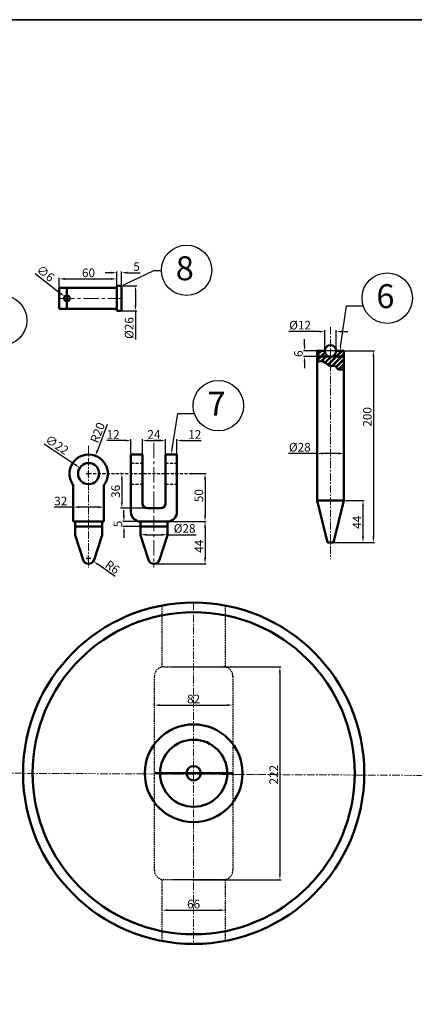
# Model space of a CAD drawing. Units: millimetres. Extents: x -282 to 2335, y -1129 to 664.
# Tile 7 of 8: x 1341 to 1752, y -363 to 664. Entities that reach past the tile are written whole.
import ezdxf
from ezdxf import colors
from ezdxf.entities.mleader import LeaderData, LeaderLine
from ezdxf.math import Vec2, Vec3

# ---------------------------------------------------------------- set-up
doc = ezdxf.new("R2010")
doc.units = ezdxf.units.MM
doc.header["$LTSCALE"] = 0.5
doc.linetypes.add('CENTER', pattern=[50.8, 31.75, -6.35, 6.35, -6.35])
doc.linetypes.add('HIDDEN', pattern=[9.525, 6.35, -3.175])
for name, color, linetype, lineweight in [('M-CNTR', 1, 'CENTER', 18), ('M-DIMS', 2, 'Continuous', 25), ('M-HATC', 8, 'Continuous', 18), ('M-HIDN', 4, 'HIDDEN', 25), ('M-OUTL', 7, 'Continuous', 50), ('M-TEXT', 3, 'Continuous', 25), ('M-TTLB', 7, 'Continuous', 35)]:
    doc.layers.add(name, color=color, linetype=linetype, lineweight=lineweight)
doc.styles.get("Standard").update_dxf_attribs({"font": 'arial.ttf'})
doc.dimstyles.new('ISO-25', dxfattribs={"dimtxt": 9, "dimasz": 6, "dimexe": 1.25, "dimexo": 0.625, "dimtad": 1, "dimtxsty": 'Standard', "dimcen": 2.5, "dimadec": 0, "dimazin": 0, "dimtfac": 1, "dimtofl": 0, "dimtmove": 0, "dimatfit": 3, "dimfxl": 1, "dimarcsym": 0})

# ---------------------------------------------------------------- blocks, each defined once
blk = doc.blocks.new('*D82')
at = {"layer": 'Defpoints', "color": 0, "transparency": 16777216}
for p in [(1442, 393.4), (1382, 384.1), (1442, 384.1)]:
    blk.add_point(p, dxfattribs=at)
at = {"layer": 'M-DIMS', "color": 0, "lineweight": -2, "transparency": 16777216}
for p, q in [((1382, 384.8), (1382, 394.6)), ((1388, 393.4), (1436, 393.4)), ((1442, 384.8), (1442, 394.6))]:
    blk.add_line(p, q, dxfattribs=at)
at = {"layer": 'M-DIMS', "color": 0, "transparency": 16777216}
for points in [[(1388, 394.4), (1388, 392.4), (1382, 393.4)], [(1436, 394.4), (1436, 392.4), (1442, 393.4)]]:
    blk.add_solid(points, dxfattribs=at)
at = {"layer": 'M-DIMS', "color": 0, "transparency": 16777216, "insert": (1412.5, 398.6), "char_height": 9, "attachment_point": 5}
blk.add_mtext('60', dxfattribs=at)
blk = doc.blocks.new('*D83')
at = {"layer": 'Defpoints', "color": 0, "transparency": 16777216}
for p in [(1447, 399.9), (1442, 386.1), (1447, 386.1)]:
    blk.add_point(p, dxfattribs=at)
at = {"layer": 'M-DIMS', "color": 0, "lineweight": -2, "transparency": 16777216}
for p, q in [((1442, 386.8), (1442, 401.2)), ((1447, 386.8), (1447, 401.2)), ((1436, 399.9), (1430, 399.9)), ((1453, 399.9), (1466.3, 399.9))]:
    blk.add_line(p, q, dxfattribs=at)
at = {"layer": 'M-DIMS', "color": 0, "transparency": 16777216}
for points in [[(1436, 400.9), (1436, 398.9), (1442, 399.9)], [(1453, 400.9), (1453, 398.9), (1447, 399.9)]]:
    blk.add_solid(points, dxfattribs=at)
at = {"layer": 'M-DIMS', "color": 0, "transparency": 16777216, "insert": (1462.7, 405.1), "char_height": 9, "attachment_point": 5}
blk.add_mtext('5', dxfattribs=at)
blk = doc.blocks.new('*D84')
at = {"layer": 'Defpoints', "color": 0, "transparency": 16777216}
for p in [(1447, 386.1), (1447, 360.1), (1461.6, 360.1)]:
    blk.add_point(p, dxfattribs=at)
at = {"layer": 'M-DIMS', "color": 0, "lineweight": -2, "transparency": 16777216}
for p, q in [((1447.7, 386.1), (1462.8, 386.1)), ((1461.6, 380.1), (1461.6, 366.1)), ((1447.7, 360.1), (1462.8, 360.1)), ((1461.6, 360.1), (1461.6, 330.2))]:
    blk.add_line(p, q, dxfattribs=at)
at = {"layer": 'M-DIMS', "color": 0, "transparency": 16777216}
for points in [[(1460.6, 380.1), (1462.6, 380.1), (1461.6, 386.1)], [(1460.6, 366.1), (1462.6, 366.1), (1461.6, 360.1)]]:
    blk.add_solid(points, dxfattribs=at)
at = {"layer": 'M-DIMS', "color": 0, "transparency": 16777216, "insert": (1456.1, 342.2), "char_height": 9, "attachment_point": 5, "rotation": 90}
blk.add_mtext('%%C26', dxfattribs=at)
blk = doc.blocks.new('*D85')
at = {"layer": 'Defpoints', "color": 0, "transparency": 16777216}
for p in [(1387.7, 375), (1392.4, 371.3)]:
    blk.add_point(p, dxfattribs=at)
at = {"layer": 'M-DIMS', "color": 0, "lineweight": -2, "transparency": 16777216}
for p, q in [((1356.9, 399.1), (1383, 378.7)), ((1387.5, 373.1), (1392.5, 373.1)), ((1390, 370.6), (1390, 375.6))]:
    blk.add_line(p, q, dxfattribs=at)
at = {"layer": 'M-DIMS', "color": 0, "transparency": 16777216}
blk.add_solid([(1383.6, 379.5), (1382.3, 377.9), (1387.7, 375)], dxfattribs=at)
at = {"layer": 'M-DIMS', "color": 0, "transparency": 16777216, "insert": (1367, 398.2), "char_height": 9, "attachment_point": 5, "rotation": 321.8983}
blk.add_mtext('∅6', dxfattribs=at)
blk = doc.blocks.new('*D86')
at = {"layer": 'Defpoints', "color": 0, "ltscale": 0.5, "transparency": 16777216}
for p in [(1403.5, 196.4), (1421.8, 184.2)]:
    blk.add_point(p, dxfattribs=at)
at = {"layer": 'M-DIMS', "color": 0, "lineweight": -2, "ltscale": 0.5, "transparency": 16777216}
for p, q in [((1366.1, 221.5), (1398.5, 199.8)), ((1410.1, 190.3), (1415.1, 190.3)), ((1412.6, 187.8), (1412.6, 192.8))]:
    blk.add_line(p, q, dxfattribs=at)
at = {"layer": 'M-DIMS', "color": 0, "ltscale": 0.5, "transparency": 16777216}
blk.add_solid([(1399.1, 200.6), (1398, 198.9), (1403.5, 196.4)], dxfattribs=at)
at = {"layer": 'M-DIMS', "color": 0, "ltscale": 0.5, "transparency": 16777216, "insert": (1379, 219.4), "char_height": 9, "attachment_point": 5, "rotation": 326.1447}
blk.add_mtext('∅22', dxfattribs=at)
blk = doc.blocks.new('*D87')
at = {"layer": 'Defpoints', "color": 0, "ltscale": 0.5, "transparency": 16777216}
for p in [(1468.8, 224.8), (1456.8, 210.3), (1468.8, 210.3)]:
    blk.add_point(p, dxfattribs=at)
at = {"layer": 'M-DIMS', "color": 0, "lineweight": -2, "ltscale": 0.5, "transparency": 16777216}
for p, q in [((1456.8, 210.9), (1456.8, 226.1)), ((1468.8, 210.9), (1468.8, 226.1)), ((1450.8, 224.8), (1431.6, 224.8)), ((1474.8, 224.8), (1480.8, 224.8))]:
    blk.add_line(p, q, dxfattribs=at)
at = {"layer": 'M-DIMS', "color": 0, "ltscale": 0.5, "transparency": 16777216}
for points in [[(1450.8, 225.8), (1450.8, 223.8), (1456.8, 224.8)], [(1474.8, 225.8), (1474.8, 223.8), (1468.8, 224.8)]]:
    blk.add_solid(points, dxfattribs=at)
at = {"layer": 'M-DIMS', "color": 0, "ltscale": 0.5, "transparency": 16777216, "insert": (1438.2, 230), "char_height": 9, "attachment_point": 5}
blk.add_mtext('12', dxfattribs=at)
blk = doc.blocks.new('*D88')
at = {"layer": 'Defpoints', "color": 0, "ltscale": 0.5, "transparency": 16777216}
for p in [(1492.8, 224.8), (1468.8, 210.3), (1492.8, 210.3)]:
    blk.add_point(p, dxfattribs=at)
at = {"layer": 'M-DIMS', "color": 0, "lineweight": -2, "ltscale": 0.5, "transparency": 16777216}
for p, q in [((1468.8, 210.9), (1468.8, 226.1)), ((1492.8, 210.9), (1492.8, 226.1)), ((1474.8, 224.8), (1486.8, 224.8))]:
    blk.add_line(p, q, dxfattribs=at)
at = {"layer": 'M-DIMS', "color": 0, "ltscale": 0.5, "transparency": 16777216}
for points in [[(1474.8, 225.8), (1474.8, 223.8), (1468.8, 224.8)], [(1486.8, 225.8), (1486.8, 223.8), (1492.8, 224.8)]]:
    blk.add_solid(points, dxfattribs=at)
at = {"layer": 'M-DIMS', "color": 0, "ltscale": 0.5, "transparency": 16777216, "insert": (1480.8, 230), "char_height": 9, "attachment_point": 5}
blk.add_mtext('24', dxfattribs=at)
blk = doc.blocks.new('*D89')
at = {"layer": 'Defpoints', "color": 0, "ltscale": 0.5, "transparency": 16777216}
for p in [(1504.8, 224.8), (1492.8, 210.3), (1504.8, 210.3)]:
    blk.add_point(p, dxfattribs=at)
at = {"layer": 'M-DIMS', "color": 0, "lineweight": -2, "ltscale": 0.5, "transparency": 16777216}
for p, q in [((1492.8, 210.9), (1492.8, 226.1)), ((1504.8, 210.9), (1504.8, 226.1)), ((1486.8, 224.8), (1480.8, 224.8)), ((1510.8, 224.8), (1530, 224.8))]:
    blk.add_line(p, q, dxfattribs=at)
at = {"layer": 'M-DIMS', "color": 0, "ltscale": 0.5, "transparency": 16777216}
for points in [[(1486.8, 225.8), (1486.8, 223.8), (1492.8, 224.8)], [(1510.8, 225.8), (1510.8, 223.8), (1504.8, 224.8)]]:
    blk.add_solid(points, dxfattribs=at)
at = {"layer": 'M-DIMS', "color": 0, "ltscale": 0.5, "transparency": 16777216, "insert": (1523.4, 230), "char_height": 9, "attachment_point": 5}
blk.add_mtext('12', dxfattribs=at)
blk = doc.blocks.new('*D90')
at = {"layer": 'Defpoints', "color": 0, "ltscale": 0.5, "transparency": 16777216}
for p in [(1447.5, 190.3), (1447.3, 154.3), (1480.8, 154.3)]:
    blk.add_point(p, dxfattribs=at)
at = {"layer": 'M-DIMS', "color": 0, "lineweight": -2, "ltscale": 0.5, "transparency": 16777216}
for p, q in [((1446.9, 190.3), (1446, 190.3)), ((1447.3, 184.3), (1447.3, 160.3)), ((1480.2, 154.3), (1446, 154.3))]:
    blk.add_line(p, q, dxfattribs=at)
at = {"layer": 'M-DIMS', "color": 0, "ltscale": 0.5, "transparency": 16777216}
for points in [[(1446.3, 184.3), (1448.3, 184.3), (1447.3, 190.3)], [(1446.3, 160.3), (1448.3, 160.3), (1447.3, 154.3)]]:
    blk.add_solid(points, dxfattribs=at)
at = {"layer": 'M-DIMS', "color": 0, "ltscale": 0.5, "transparency": 16777216, "insert": (1442, 171.8), "char_height": 9, "attachment_point": 5, "rotation": 90}
blk.add_mtext('36', dxfattribs=at)
blk = doc.blocks.new('*D91')
at = {"layer": 'Defpoints', "color": 0, "ltscale": 0.5, "transparency": 16777216}
for p in [(1449.5, 135.3), (1466.8, 140.3), (1466.8, 135.3)]:
    blk.add_point(p, dxfattribs=at)
at = {"layer": 'M-DIMS', "color": 0, "lineweight": -2, "ltscale": 0.5, "transparency": 16777216}
for p, q in [((1449.5, 146.3), (1449.5, 152.3)), ((1466.2, 140.3), (1448.3, 140.3)), ((1466.2, 135.3), (1448.3, 135.3)), ((1449.5, 129.3), (1449.5, 123.3))]:
    blk.add_line(p, q, dxfattribs=at)
at = {"layer": 'M-DIMS', "color": 0, "ltscale": 0.5, "transparency": 16777216}
for points in [[(1448.5, 146.3), (1450.5, 146.3), (1449.5, 140.3)], [(1448.5, 129.3), (1450.5, 129.3), (1449.5, 135.3)]]:
    blk.add_solid(points, dxfattribs=at)
at = {"layer": 'M-DIMS', "color": 0, "ltscale": 0.5, "transparency": 16777216, "insert": (1444.3, 137.8), "char_height": 9, "attachment_point": 5, "rotation": 90}
blk.add_mtext('5', dxfattribs=at)
blk = doc.blocks.new('*D92')
at = {"layer": 'Defpoints', "color": 0, "ltscale": 0.5, "transparency": 16777216}
for p in [(1396.6, 155.7), (1428.6, 155.7), (1428.6, 155.4)]:
    blk.add_point(p, dxfattribs=at)
at = {"layer": 'M-DIMS', "color": 0, "lineweight": -2, "ltscale": 0.5, "transparency": 16777216}
for p, q in [((1396.6, 155.4), (1376.6, 155.4)), ((1396.6, 155), (1396.6, 154.1)), ((1422.6, 155.4), (1402.6, 155.4)), ((1428.6, 155), (1428.6, 154.1))]:
    blk.add_line(p, q, dxfattribs=at)
at = {"layer": 'M-DIMS', "color": 0, "ltscale": 0.5, "transparency": 16777216}
for points in [[(1402.6, 156.4), (1402.6, 154.4), (1396.6, 155.4)], [(1422.6, 156.4), (1422.6, 154.4), (1428.6, 155.4)]]:
    blk.add_solid(points, dxfattribs=at)
at = {"layer": 'M-DIMS', "color": 0, "ltscale": 0.5, "transparency": 16777216, "insert": (1383.6, 160.6), "char_height": 9, "attachment_point": 5}
blk.add_mtext('32', dxfattribs=at)
blk = doc.blocks.new('*D93')
at = {"layer": 'Defpoints', "color": 0, "ltscale": 0.5, "transparency": 16777216}
for p in [(1480.8, 140.3), (1480.8, 96.3), (1534.1, 96.3)]:
    blk.add_point(p, dxfattribs=at)
at = {"layer": 'M-DIMS', "color": 0, "lineweight": -2, "ltscale": 0.5, "transparency": 16777216}
for p, q in [((1481.5, 140.3), (1535.3, 140.3)), ((1534.1, 134.3), (1534.1, 102.3)), ((1481.5, 96.3), (1535.3, 96.3))]:
    blk.add_line(p, q, dxfattribs=at)
at = {"layer": 'M-DIMS', "color": 0, "ltscale": 0.5, "transparency": 16777216}
for points in [[(1533.1, 134.3), (1535.1, 134.3), (1534.1, 140.3)], [(1533.1, 102.3), (1535.1, 102.3), (1534.1, 96.3)]]:
    blk.add_solid(points, dxfattribs=at)
at = {"layer": 'M-DIMS', "color": 0, "ltscale": 0.5, "transparency": 16777216, "insert": (1528.9, 114.6), "char_height": 9, "attachment_point": 5, "rotation": 90}
blk.add_mtext('44', dxfattribs=at)
blk = doc.blocks.new('*D94')
at = {"layer": 'Defpoints', "color": 0, "ltscale": 0.5, "transparency": 16777216}
for p in [(1519.3, 190.3), (1508.4, 140.3), (1534.1, 140.3)]:
    blk.add_point(p, dxfattribs=at)
at = {"layer": 'M-DIMS', "color": 0, "lineweight": -2, "ltscale": 0.5, "transparency": 16777216}
for p, q in [((1519.9, 190.3), (1535.3, 190.3)), ((1534.1, 184.3), (1534.1, 146.3)), ((1509, 140.3), (1535.3, 140.3))]:
    blk.add_line(p, q, dxfattribs=at)
at = {"layer": 'M-DIMS', "color": 0, "ltscale": 0.5, "transparency": 16777216}
for points in [[(1533.1, 184.3), (1535.1, 184.3), (1534.1, 190.3)], [(1533.1, 146.3), (1535.1, 146.3), (1534.1, 140.3)]]:
    blk.add_solid(points, dxfattribs=at)
at = {"layer": 'M-DIMS', "color": 0, "ltscale": 0.5, "transparency": 16777216, "insert": (1528.8, 167.3), "char_height": 9, "attachment_point": 5, "rotation": 90}
blk.add_mtext('50', dxfattribs=at)
blk = doc.blocks.new('*D95')
at = {"layer": 'Defpoints', "color": 0, "ltscale": 0.5, "transparency": 16777216}
for p in [(1419.7, 209), (1412.6, 190.3)]:
    blk.add_point(p, dxfattribs=at)
at = {"layer": 'M-DIMS', "color": 0, "lineweight": -2, "ltscale": 0.5, "transparency": 16777216}
for p, q in [((1432, 241.5), (1421.9, 214.6)), ((1410.1, 190.3), (1415.1, 190.3)), ((1412.6, 187.8), (1412.6, 192.8))]:
    blk.add_line(p, q, dxfattribs=at)
at = {"layer": 'M-DIMS', "color": 0, "ltscale": 0.5, "transparency": 16777216}
blk.add_solid([(1420.9, 215), (1422.8, 214.3), (1419.7, 209)], dxfattribs=at)
at = {"layer": 'M-DIMS', "color": 0, "ltscale": 0.5, "transparency": 16777216, "insert": (1423.1, 232.7), "char_height": 9, "attachment_point": 5, "rotation": 69.2216}
blk.add_mtext('R20', dxfattribs=at)
blk = doc.blocks.new('*D96')
at = {"layer": 'Defpoints', "color": 0, "ltscale": 0.5, "transparency": 16777216}
for p in [(1412.6, 102.3), (1417.6, 98.9)]:
    blk.add_point(p, dxfattribs=at)
at = {"layer": 'M-DIMS', "color": 0, "lineweight": -2, "ltscale": 0.5, "transparency": 16777216}
for p, q in [((1412.6, 99.8), (1412.6, 104.8)), ((1410.1, 102.3), (1415.1, 102.3)), ((1440.3, 83), (1422.5, 95.4))]:
    blk.add_line(p, q, dxfattribs=at)
at = {"layer": 'M-DIMS', "color": 0, "ltscale": 0.5, "transparency": 16777216}
blk.add_solid([(1423, 96.2), (1421.9, 94.6), (1417.6, 98.9)], dxfattribs=at)
at = {"layer": 'M-DIMS', "color": 0, "ltscale": 0.5, "transparency": 16777216, "insert": (1436.8, 91.8), "char_height": 9, "attachment_point": 5, "rotation": 325.0622}
blk.add_mtext('R6', dxfattribs=at)
blk = doc.blocks.new('*D97')
at = {"layer": 'Defpoints', "color": 0, "ltscale": 0.5, "transparency": 16777216}
for p in [(1466.8, 126), (1494.8, 126.6), (1494.8, 126)]:
    blk.add_point(p, dxfattribs=at)
at = {"layer": 'M-DIMS', "color": 0, "lineweight": -2, "ltscale": 0.5, "transparency": 16777216}
for p, q in [((1466.8, 126.6), (1466.8, 127.8)), ((1472.8, 126.6), (1488.8, 126.6)), ((1494.8, 126.6), (1494.8, 127.8)), ((1494.8, 126.6), (1524.8, 126.6))]:
    blk.add_line(p, q, dxfattribs=at)
at = {"layer": 'M-DIMS', "color": 0, "ltscale": 0.5, "transparency": 16777216}
for points in [[(1472.8, 127.6), (1472.8, 125.6), (1466.8, 126.6)], [(1488.8, 127.6), (1488.8, 125.6), (1494.8, 126.6)]]:
    blk.add_solid(points, dxfattribs=at)
at = {"layer": 'M-DIMS', "color": 0, "ltscale": 0.5, "transparency": 16777216, "insert": (1512.8, 132), "char_height": 9, "attachment_point": 5}
blk.add_mtext('%%C28', dxfattribs=at)
blk = doc.blocks.new('*D110')
at = {"layer": 'Defpoints', "color": 0, "ltscale": 0.5, "transparency": 16777216}
for p in [(1522.2, -11.2), (1522.2, -233.2), (1612.2, -233.2)]:
    blk.add_point(p, dxfattribs=at)
at = {"layer": 'M-DIMS', "color": 0, "lineweight": -2, "ltscale": 0.5, "transparency": 16777216}
for p, q in [((1522.9, -11.2), (1613.4, -11.2)), ((1612.2, -17.2), (1612.2, -227.2)), ((1522.9, -233.2), (1613.4, -233.2))]:
    blk.add_line(p, q, dxfattribs=at)
at = {"layer": 'M-DIMS', "color": 0, "ltscale": 0.5, "transparency": 16777216}
for points in [[(1611.2, -17.2), (1613.2, -17.2), (1612.2, -11.2)], [(1611.2, -227.2), (1613.2, -227.2), (1612.2, -233.2)]]:
    blk.add_solid(points, dxfattribs=at)
at = {"layer": 'M-DIMS', "color": 0, "ltscale": 0.5, "transparency": 16777216, "insert": (1607, -123.7), "char_height": 9, "attachment_point": 5, "rotation": 90}
blk.add_mtext('222', dxfattribs=at)
blk = doc.blocks.new('*D111')
at = {"layer": 'Defpoints', "color": 0, "ltscale": 0.5, "transparency": 16777216}
for p in [(1481.2, -51.1), (1563.2, -51.1), (1563.2, -51.1)]:
    blk.add_point(p, dxfattribs=at)
at = {"layer": 'M-DIMS', "color": 0, "lineweight": -2, "ltscale": 0.5, "transparency": 16777216}
for p, q in [((1481.2, -50.5), (1481.2, -49.8)), ((1487.2, -51.1), (1557.2, -51.1)), ((1563.2, -50.5), (1563.2, -49.8))]:
    blk.add_line(p, q, dxfattribs=at)
at = {"layer": 'M-DIMS', "color": 0, "ltscale": 0.5, "transparency": 16777216}
for points in [[(1487.2, -50.1), (1487.2, -52.1), (1481.2, -51.1)], [(1557.2, -50.1), (1557.2, -52.1), (1563.2, -51.1)]]:
    blk.add_solid(points, dxfattribs=at)
at = {"layer": 'M-DIMS', "color": 0, "ltscale": 0.5, "transparency": 16777216, "insert": (1522.2, -45.9), "char_height": 9, "attachment_point": 5}
blk.add_mtext('82', dxfattribs=at)
blk = doc.blocks.new('*D112')
at = {"layer": 'Defpoints', "color": 0, "ltscale": 0.5, "transparency": 16777216}
for p in [(1489.2, -265), (1555.2, -265), (1555.2, -265)]:
    blk.add_point(p, dxfattribs=at)
at = {"layer": 'M-DIMS', "color": 0, "lineweight": -2, "ltscale": 0.5, "transparency": 16777216}
for p, q in [((1489.2, -264.4), (1489.2, -263.8)), ((1495.2, -265), (1549.2, -265)), ((1555.2, -264.4), (1555.2, -263.8))]:
    blk.add_line(p, q, dxfattribs=at)
at = {"layer": 'M-DIMS', "color": 0, "ltscale": 0.5, "transparency": 16777216}
for points in [[(1495.2, -264), (1495.2, -266), (1489.2, -265)], [(1549.2, -264), (1549.2, -266), (1555.2, -265)]]:
    blk.add_solid(points, dxfattribs=at)
at = {"layer": 'M-DIMS', "color": 0, "ltscale": 0.5, "transparency": 16777216, "insert": (1522.2, -259.8), "char_height": 9, "attachment_point": 5}
blk.add_mtext('66', dxfattribs=at)
blk = doc.blocks.new('*D113')
at = {"layer": 'Defpoints', "color": 0, "ltscale": 0.5, "transparency": 16777216}
for p in [(1679, 211.3), (1651, 196), (1679, 196)]:
    blk.add_point(p, dxfattribs=at)
at = {"layer": 'M-DIMS', "color": 0, "lineweight": -2, "ltscale": 0.5, "transparency": 16777216}
for p, q in [((1651, 211.3), (1621.1, 211.3)), ((1651, 196.6), (1651, 212.5)), ((1673, 211.3), (1657, 211.3)), ((1679, 196.6), (1679, 212.5))]:
    blk.add_line(p, q, dxfattribs=at)
at = {"layer": 'M-DIMS', "color": 0, "ltscale": 0.5, "transparency": 16777216}
for points in [[(1657, 212.3), (1657, 210.3), (1651, 211.3)], [(1673, 212.3), (1673, 210.3), (1679, 211.3)]]:
    blk.add_solid(points, dxfattribs=at)
at = {"layer": 'M-DIMS', "color": 0, "ltscale": 0.5, "transparency": 16777216, "insert": (1633, 216.7), "char_height": 9, "attachment_point": 5}
blk.add_mtext('%%C28', dxfattribs=at)
blk = doc.blocks.new('*D114')
at = {"layer": 'Defpoints', "color": 0, "ltscale": 0.5, "transparency": 16777216}
for p in [(1671, 338.5), (1659, 318.4), (1671, 318.4)]:
    blk.add_point(p, dxfattribs=at)
at = {"layer": 'M-DIMS', "color": 0, "lineweight": -2, "ltscale": 0.5, "transparency": 16777216}
for p, q in [((1659, 319.1), (1659, 339.8)), ((1671, 319.1), (1671, 339.8)), ((1653, 338.5), (1621.4, 338.5)), ((1677, 338.5), (1683, 338.5))]:
    blk.add_line(p, q, dxfattribs=at)
at = {"layer": 'M-DIMS', "color": 0, "ltscale": 0.5, "transparency": 16777216}
for points in [[(1653, 339.5), (1653, 337.5), (1659, 338.5)], [(1677, 339.5), (1677, 337.5), (1671, 338.5)]]:
    blk.add_solid(points, dxfattribs=at)
at = {"layer": 'M-DIMS', "color": 0, "ltscale": 0.5, "transparency": 16777216, "insert": (1633.3, 344), "char_height": 9, "attachment_point": 5}
blk.add_mtext('%%C12', dxfattribs=at)
blk = doc.blocks.new('*D115')
at = {"layer": 'Defpoints', "color": 0, "ltscale": 0.5, "transparency": 16777216}
for p in [(1679, 318.4), (1637.9, 312.4), (1679, 312.4)]:
    blk.add_point(p, dxfattribs=at)
at = {"layer": 'M-DIMS', "color": 0, "lineweight": -2, "ltscale": 0.5, "transparency": 16777216}
for p, q in [((1637.9, 324.4), (1637.9, 330.4)), ((1678.4, 318.4), (1636.7, 318.4)), ((1678.4, 312.4), (1636.7, 312.4)), ((1637.9, 306.4), (1637.9, 300.4))]:
    blk.add_line(p, q, dxfattribs=at)
at = {"layer": 'M-DIMS', "color": 0, "ltscale": 0.5, "transparency": 16777216}
for points in [[(1636.9, 324.4), (1638.9, 324.4), (1637.9, 318.4)], [(1636.9, 306.4), (1638.9, 306.4), (1637.9, 312.4)]]:
    blk.add_solid(points, dxfattribs=at)
at = {"layer": 'M-DIMS', "color": 0, "ltscale": 0.5, "transparency": 16777216, "insert": (1632.7, 315.4), "char_height": 9, "attachment_point": 5, "rotation": 90}
blk.add_mtext('6', dxfattribs=at)
blk = doc.blocks.new('*D116')
at = {"layer": 'Defpoints', "color": 0, "ltscale": 0.5, "transparency": 16777216}
for p in [(1679, 318.4), (1666.5, 118.4), (1709.8, 118.4)]:
    blk.add_point(p, dxfattribs=at)
at = {"layer": 'M-DIMS', "color": 0, "lineweight": -2, "ltscale": 0.5, "transparency": 16777216}
for p, q in [((1679.6, 318.4), (1711.1, 318.4)), ((1709.8, 312.4), (1709.8, 124.4)), ((1667.1, 118.4), (1711.1, 118.4))]:
    blk.add_line(p, q, dxfattribs=at)
at = {"layer": 'M-DIMS', "color": 0, "ltscale": 0.5, "transparency": 16777216}
for points in [[(1708.8, 312.4), (1710.8, 312.4), (1709.8, 318.4)], [(1708.8, 124.4), (1710.8, 124.4), (1709.8, 118.4)]]:
    blk.add_solid(points, dxfattribs=at)
at = {"layer": 'M-DIMS', "color": 0, "ltscale": 0.5, "transparency": 16777216, "insert": (1704.6, 249.5), "char_height": 9, "attachment_point": 5, "rotation": 90}
blk.add_mtext('200', dxfattribs=at)
blk = doc.blocks.new('*D117')
at = {"layer": 'Defpoints', "color": 0, "ltscale": 0.5, "transparency": 16777216}
for p in [(1679, 162.4), (1662, 118.4), (1698.9, 118.4)]:
    blk.add_point(p, dxfattribs=at)
at = {"layer": 'M-DIMS', "color": 0, "lineweight": -2, "ltscale": 0.5, "transparency": 16777216}
for p, q in [((1679.6, 162.4), (1700.2, 162.4)), ((1698.9, 156.4), (1698.9, 124.4)), ((1662.6, 118.4), (1700.2, 118.4))]:
    blk.add_line(p, q, dxfattribs=at)
at = {"layer": 'M-DIMS', "color": 0, "ltscale": 0.5, "transparency": 16777216}
for points in [[(1697.9, 156.4), (1699.9, 156.4), (1698.9, 162.4)], [(1697.9, 124.4), (1699.9, 124.4), (1698.9, 118.4)]]:
    blk.add_solid(points, dxfattribs=at)
at = {"layer": 'M-DIMS', "color": 0, "ltscale": 0.5, "transparency": 16777216, "insert": (1693.8, 139.6), "char_height": 9, "attachment_point": 5, "rotation": 90}
blk.add_mtext('44', dxfattribs=at)

msp = doc.modelspace()

# ---------------------------------------------------------------- hatches: boundary and pattern name
at = {"layer": 'M-HATC', "ltscale": 0.5}
h = msp.add_hatch(dxfattribs=at)
h.set_pattern_fill('ANSI32', color=256, scale=0.4)
h.set_pattern_definition([(45, (-51.533, -51.533), (-2.694077, 2.694077), []), (45, (-49.737, -51.533), (-2.694077, 2.694077), [])])
edge = h.paths.add_edge_path()
edge.add_line((1679.009, 312.437), (1665.009, 312.437))
edge.add_line((1665.009, 312.437), (1665.009, 302.471))
edge.add_spline(control_points=[(1665.009, 302.471), (1666.563, 302.302), (1670.132, 303.771), (1672.778, 297.803), (1676.703, 298.806), (1679.009, 299.396)], knot_values=[15.33938429, 15.33938429, 15.33938429, 15.33938429, 20.0702224, 24.41922814, 30.61317858, 30.61317858, 30.61317858, 30.61317858], degree=3, periodic=0)
edge.add_line((1679.009, 299.396), (1679.009, 312.437))
edge = h.paths.add_edge_path()
edge.add_line((1665.009, 312.437), (1651.009, 312.437))
edge.add_line((1651.009, 312.437), (1651.009, 306.942))
edge.add_spline(control_points=[(1651.009, 306.942), (1653.568, 307.444), (1659.013, 308.512), (1662.34, 302.761), (1665.009, 302.471)], knot_values=[0, 0, 0, 0, 7.20755862, 15.33938429, 15.33938429, 15.33938429, 15.33938429], degree=3, periodic=0)
edge.add_line((1665.009, 302.471), (1665.009, 312.437))
h.paths.add_polyline_path([(1659.009, 318.437), (1651.009, 318.437), (1651.009, 312.437), (1665.009, 312.437, -0.41421356)])
h.paths.add_polyline_path([(1679.009, 318.437), (1671.009, 318.437, -0.41421356), (1665.009, 312.437), (1679.009, 312.437)])

# ---------------------------------------------------------------- linework, layer by layer
at = {"layer": 'M-CNTR'}
for p, q in [((1382.049, 373.138), (1447.049, 373.138)), ((1480.828, 222.359), (1480.828, 92.311))]:
    msp.add_line(p, q, dxfattribs=at)
at = {"layer": 'M-CNTR', "ltscale": 0.5}
for p, q in [((1665.009, 343.197), (1665.009, 101.025)), ((1412.632, 219.24), (1412.632, 91.942)), ((1522.238, 55.816), (1522.238, -300.184)), ((1246.826, -121.76), (2085.572, -126.112))]:
    msp.add_line(p, q, dxfattribs=at)
at = {"layer": 'M-HIDN'}
for p, q in [((1456.828, 201.3), (1468.828, 201.3)), ((1492.828, 201.3), (1504.828, 201.3)), ((1412.632, 190.3), (1532.555, 190.3)), ((1456.828, 179.3), (1468.828, 179.3)), ((1492.828, 179.3), (1504.828, 179.3))]:
    msp.add_line(p, q, dxfattribs=at)
at = {"layer": 'M-HIDN', "ltscale": 0.5}
for p, q in [((1489.238, -11.386), (1489.238, 52.73)), ((1555.238, 52.73), (1555.238, -11.386)), ((1491.238, -11.184), (1553.238, -11.184)), ((1499.238, -11.184), (1545.238, -11.184)), ((1481.238, -223.184), (1481.238, -21.184)), ((1563.238, -21.184), (1563.238, -223.184)), ((1489.238, -297.098), (1489.238, -232.982)), ((1553.238, -233.184), (1491.238, -233.184)), ((1545.238, -233.184), (1499.238, -233.184)), ((1555.238, -232.982), (1555.238, -297.098))]:
    msp.add_line(p, q, dxfattribs=at)
for centre, start, end in [((1491.238, -21.184), 90, 180), ((1553.238, -21.184), 0, 90), ((1491.238, -223.184), 180, 270), ((1553.238, -223.184), 270, 0)]:
    msp.add_arc(centre, 10, start, end, dxfattribs=at)
at = {"layer": 'M-OUTL'}
for p, q in [((1382.049, 384.138), (1442.049, 384.138)), ((1382.049, 362.138), (1382.049, 384.138)), ((1390.049, 362.138), (1390.049, 384.138)), ((1442.049, 373.138), (1442.049, 386.138)), ((1442.049, 386.138), (1447.049, 386.138)), ((1442.049, 384.138), (1442.049, 362.138)), ((1447.049, 386.138), (1447.049, 360.138)), ((1442.049, 362.138), (1382.049, 362.138)), ((1442.049, 360.138), (1442.049, 362.138)), ((1447.049, 360.138), (1442.049, 360.138)), ((1456.828, 210.3), (1468.828, 210.3)), ((1456.828, 210.3), (1456.828, 150.3)), ((1468.828, 210.3), (1468.828, 159.3)), ((1492.828, 210.3), (1492.828, 159.3)), ((1492.828, 210.3), (1504.828, 210.3)), ((1504.828, 210.3), (1504.828, 150.3)), ((1473.828, 154.3), (1487.828, 154.3)), ((1398.632, 140.3), (1398.632, 126.001)), ((1398.632, 135.3), (1426.632, 135.3)), ((1398.632, 135.3), (1426.632, 135.3)), ((1426.632, 140.3), (1426.632, 126.001)), ((1466.828, 140.3), (1466.828, 135.3)), ((1466.828, 135.3), (1494.828, 135.3)), ((1466.828, 135.3), (1494.828, 135.3)), ((1466.828, 135.3), (1494.828, 135.3)), ((1466.828, 135.3), (1466.828, 126.001)), ((1494.828, 140.3), (1494.828, 135.3)), ((1494.828, 135.3), (1494.828, 126.001))]:
    msp.add_line(p, q, dxfattribs=at)
at = {"layer": 'M-OUTL', "ltscale": 0.5}
for p, q in [((1651.009, 318.437), (1651.009, 162.437)), ((1659.009, 318.437), (1651.009, 318.437)), ((1679.009, 318.437), (1671.009, 318.437)), ((1679.009, 162.437), (1679.009, 318.437)), ((1679.009, 312.437), (1651.009, 312.437)), ((1396.632, 178.3), (1396.632, 140.3)), ((1428.632, 178.3), (1428.632, 140.3)), ((1651.009, 162.437), (1679.009, 162.437)), ((1651.009, 162.437), (1662.009, 118.437)), ((1679.009, 162.437), (1668.009, 118.437)), ((1396.632, 140.3), (1428.632, 140.3)), ((1426.632, 135.3), (1398.632, 135.3)), ((1466.828, 140.3), (1494.828, 140.3)), ((1494.828, 135.3), (1466.828, 135.3)), ((1406.925, 100.448), (1398.632, 126.001)), ((1418.339, 100.448), (1426.632, 126.001)), ((1475.121, 100.448), (1466.828, 126.001)), ((1486.535, 100.448), (1494.828, 126.001)), ((1665.009, 118.437), (1662.009, 118.437)), ((1665.009, 118.437), (1668.009, 118.437)), ((1481.238, -122.184), (1563.238, -122.184))]:
    msp.add_line(p, q, dxfattribs=at)
at = {"layer": 'M-OUTL'}
for centre, radius in [((1390.049, 373.138), 3), ((1412.632, 190.3), 11)]:
    msp.add_circle(centre, radius, dxfattribs=at)
at = {"layer": 'M-OUTL', "ltscale": 0.5}
for centre, radius in [((1665.009, 318.437), 6), ((1522.238, -122.184), 178), ((1522.238, -122.184), 168), ((1522.238, -122.184), 51), ((1522.238, -122.184), 35), ((1522.238, -122.184), 7.5)]:
    msp.add_circle(centre, radius, dxfattribs=at)
at = {"layer": 'M-OUTL'}
for centre, radius, start, end in [((1412.632, 190.3), 20, 323.130102, 216.869898), ((1473.828, 159.3), 5, 180, 270), ((1487.828, 159.3), 5, 270, 360)]:
    msp.add_arc(centre, radius, start, end, dxfattribs=at)
at = {"layer": 'M-OUTL', "ltscale": 0.5}
for centre, radius, start, end in [((1466.828, 150.3), 10, 180, 270), ((1494.828, 150.3), 10, 270, 0), ((1412.632, 102.3), 6, 197.980672, 342.019328), ((1480.828, 102.3), 6, 197.980672, 342.019328)]:
    msp.add_arc(centre, radius, start, end, dxfattribs=at)
msp.add_open_spline([(1651.009, 306.942), (1653.568, 307.444), (1659.013, 308.512), (1663.366, 300.987), (1670.132, 303.771), (1672.778, 297.803), (1676.703, 298.806), (1679.009, 299.396)], degree=3, knots=[0, 0, 0, 0, 7.20755862, 15.33938429, 20.0702224, 24.41922814, 30.61317858, 30.61317858, 30.61317858, 30.61317858], dxfattribs=at)
at = {"layer": 'M-TEXT'}
for centre in [(1514.833, 402.451), (1724.172, 373.358), (1322.035, 350.242), (1547.991, 261.222)]:
    msp.add_circle(centre, 26.287, dxfattribs=at)
at = {"layer": 'M-TTLB', "ltscale": 0.5}
msp.add_lwpolyline([(-281.776, 663.767), (2334.915, 663.767), (2334.915, -1128.523), (-281.776, -1128.523)], close=True, dxfattribs=at)

# ---------------------------------------------------------------- texts
at = {"layer": 'M-TEXT', "char_height": 25, "attachment_point": 1}
for s, insert in [('\\pxqc;8', (1500.5, 416.992)), ('\\pxqc;6', (1709.839, 387.898)), ('\\pxqc;7', (1533.658, 275.762))]:
    msp.add_mtext_dynamic_manual_height_columns(s, width=25, gutter_width=12.5, heights=[7.196], dxfattribs=dict(at, insert=insert))

# ---------------------------------------------------------------- dimensions: what is measured, and where the dimension line sits
at = {"layer": 'M-DIMS'}
for base, p1, p2, picture, middle in [((1447.049, 399.945), (1442.049, 386.138), (1447.049, 386.138), '*D83', (1462.657, 399.945)), ((1442.049, 393.371), (1382.049, 384.138), (1442.049, 384.138), '*D82', (1412.468, 393.371))]:
    dim = msp.add_linear_dim(base=base, p1=p1, p2=p2, dimstyle='ISO-25', override={"dimclrd": 0, "dimclre": 0, "dimclrt": 0}, dxfattribs=at)
    dim.commit()
    dim.dimension.update_dxf_attribs({"geometry": picture, "text_midpoint": middle, "dimtype": 160})
dim = msp.add_diameter_dim_2p(p1=(1392.41, 371.287), p2=(1387.688, 374.989), dimstyle='ISO-25', override={"dimclrd": 0, "dimclre": 0, "dimclrt": 0}, dxfattribs=at)
dim.commit()
dim.dimension.update_dxf_attribs({"geometry": '*D85', "text_midpoint": (1363.605, 393.874), "dimtype": 163})
dim = msp.add_linear_dim(base=(1461.558, 360.138), p1=(1447.049, 386.138), p2=(1447.049, 360.138), angle=90, text='%%C<>', dimstyle='ISO-25', override={"dimclrd": 0, "dimclre": 0, "dimclrt": 0}, dxfattribs=at)
dim.commit()
dim.dimension.update_dxf_attribs({"geometry": '*D84', "text_midpoint": (1461.558, 342.174), "dimtype": 160})
at = {"layer": 'M-DIMS', "ltscale": 0.5}
for base, p1, p2, picture, middle in [((1671.009, 338.518), (1659.009, 318.437), (1671.009, 318.437), '*D114', (1633.337, 338.518)), ((1679.009, 211.263), (1651.009, 195.999), (1679.009, 195.999), '*D113', (1633.033, 211.263)), ((1494.828, 126.553), (1466.828, 126.001), (1494.828, 126.001), '*D97', (1512.805, 126.553))]:
    dim = msp.add_linear_dim(base=base, p1=p1, p2=p2, text='%%C<>', dimstyle='ISO-25', override={"dimclrd": 0, "dimclre": 0, "dimclrt": 0}, dxfattribs=at)
    dim.commit()
    dim.dimension.update_dxf_attribs({"geometry": picture, "text_midpoint": middle, "dimtype": 160})
for base, p1, p2, picture, middle in [((1637.929, 312.437), (1679.009, 318.437), (1679.009, 312.437), '*D115', (1637.929, 315.437)), ((1709.829, 118.437), (1679.009, 318.437), (1666.509, 118.437), '*D116', (1709.829, 249.485)), ((1447.271, 154.3), (1447.492, 190.3), (1480.828, 154.3), '*D90', (1447.271, 171.758)), ((1534.053, 140.3), (1519.302, 190.3), (1508.378, 140.3), '*D94', (1534.053, 167.282)), ((1698.939, 118.437), (1679.009, 162.437), (1662.009, 118.437), '*D117', (1698.939, 139.575)), ((1449.546, 135.3), (1466.828, 140.3), (1466.828, 135.3), '*D91', (1449.546, 137.8)), ((1534.053, 96.3), (1480.828, 140.3), (1480.828, 96.3), '*D93', (1534.053, 114.633)), ((1612.186, -233.184), (1522.238, -11.184), (1522.238, -233.184), '*D110', (1612.186, -123.656))]:
    dim = msp.add_linear_dim(base=base, p1=p1, p2=p2, angle=90, dimstyle='ISO-25', override={"dimclrd": 0, "dimclre": 0, "dimclrt": 0}, dxfattribs=at)
    dim.commit()
    dim.dimension.update_dxf_attribs({"geometry": picture, "text_midpoint": middle, "dimtype": 160})
for center, mpoint, picture, middle in [((1412.632, 190.3), (1419.727, 209), '*D95', (1423.135, 232.694)), ((1412.632, 102.3), (1417.551, 98.864), '*D96', (1436.836, 91.76))]:
    dim = msp.add_radius_dim(center=center, mpoint=mpoint, dimstyle='ISO-25', override={"dimclrd": 0, "dimclre": 0, "dimclrt": 0}, dxfattribs=at)
    dim.commit()
    dim.dimension.update_dxf_attribs({"geometry": picture, "text_midpoint": middle})
dim = msp.add_diameter_dim_2p(p1=(1421.767, 184.172), p2=(1403.497, 196.429), dimstyle='ISO-25', override={"dimclrd": 0, "dimclre": 0, "dimclrt": 0}, dxfattribs=at)
dim.commit()
dim.dimension.update_dxf_attribs({"geometry": '*D86', "text_midpoint": (1375.962, 214.901), "dimtype": 163})
for base, p1, p2, picture, middle in [((1468.828, 224.816), (1456.828, 210.3), (1468.828, 210.3), '*D87', (1438.227, 224.816)), ((1492.828, 224.816), (1468.828, 210.3), (1492.828, 210.3), '*D88', (1480.828, 224.816)), ((1504.828, 224.816), (1492.828, 210.3), (1504.828, 210.3), '*D89', (1523.43, 224.816)), ((1428.632, 155.39), (1396.632, 155.667), (1428.632, 155.667), '*D92', (1383.61, 155.39)), ((1563.238, -51.1), (1481.238, -51.1), (1563.238, -51.1), '*D111', (1522.238, -51.1)), ((1555.238, -265.04), (1489.238, -265.04), (1555.238, -265.04), '*D112', (1522.238, -265.04))]:
    dim = msp.add_linear_dim(base=base, p1=p1, p2=p2, dimstyle='ISO-25', override={"dimclrd": 0, "dimclre": 0, "dimclrt": 0}, dxfattribs=at)
    dim.commit()
    dim.dimension.update_dxf_attribs({"geometry": picture, "text_midpoint": middle, "dimtype": 160})

# ---------------------------------------------------------------- leaders
at = {"layer": 'M-TEXT', "ltscale": 0.5}
ml = msp.add_multileader_mtext('Standard', dxfattribs=at)
ml.set_content(' ', color=256)
ml.set_leader_properties()
ml.build(insert=Vec2(0, 0))
ctx = ml.context
ctx.base_point, ctx.plane_origin = Vec3(1488.548, 402.082), Vec3(1447.049, 386.138)
notes = []
notes.append((ctx, [(0, (1, 1, 0), (1480.548, 402.082), (1, 0), 8, [(0, [(1447.049, 386.138)], 0, [])])]))
ctx.mtext.insert, ctx.mtext.flow_direction = Vec3(1490.548, 404.082), 5
ml = msp.add_multileader_mtext('Standard', dxfattribs=at)
ml.set_content('', color=256)
ml.set_leader_properties()
ml.build(insert=Vec2(0, 0))
ctx = ml.context
ctx.base_point, ctx.plane_origin = Vec3(1699.052, 365.251), Vec3(1675.009, 322.437)
notes.append((ctx, [(0, (1, 1, 0), (1681.778, 365.251), (1, 0), 17.275, [(0, [(1675.009, 318.437)], 0, [])])]))
ctx.mtext.insert, ctx.mtext.flow_direction = Vec3(1701.052, 367.251), 5
ml = msp.add_multileader_mtext('Standard', dxfattribs=at)
ml.set_content('', color=256)
ml.set_leader_properties()
ml.build(insert=Vec2(0, 0))
ctx = ml.context
ctx.base_point, ctx.plane_origin = Vec3(1522.871, 253.114), Vec3(1498.828, 210.3)
notes.append((ctx, [(0, (1, 1, 0), (1505.596, 253.114), (1, 0), 17.275, [(0, [(1498.828, 210.3)], 0, [])])]))
ctx.mtext.insert, ctx.mtext.flow_direction = Vec3(1524.871, 255.114), 5
for ctx, leaders in notes:
    for number, flags, end, landing, length, lines in leaders:
        leader = LeaderData()
        leader.index, (leader.has_last_leader_line, leader.has_dogleg_vector, leader.attachment_direction) = number, flags
        leader.last_leader_point, leader.dogleg_vector, leader.dogleg_length = Vec3(end), Vec3(landing), length
        for number, points, colour, breaks in lines:
            line = LeaderLine()
            line.index, line.vertices, line.color, line.breaks = number, Vec3.list(points), colors.encode_raw_color(colour), breaks
            leader.lines.append(line)
        ctx.leaders.append(leader)

doc.saveas('drawing.dxf')
